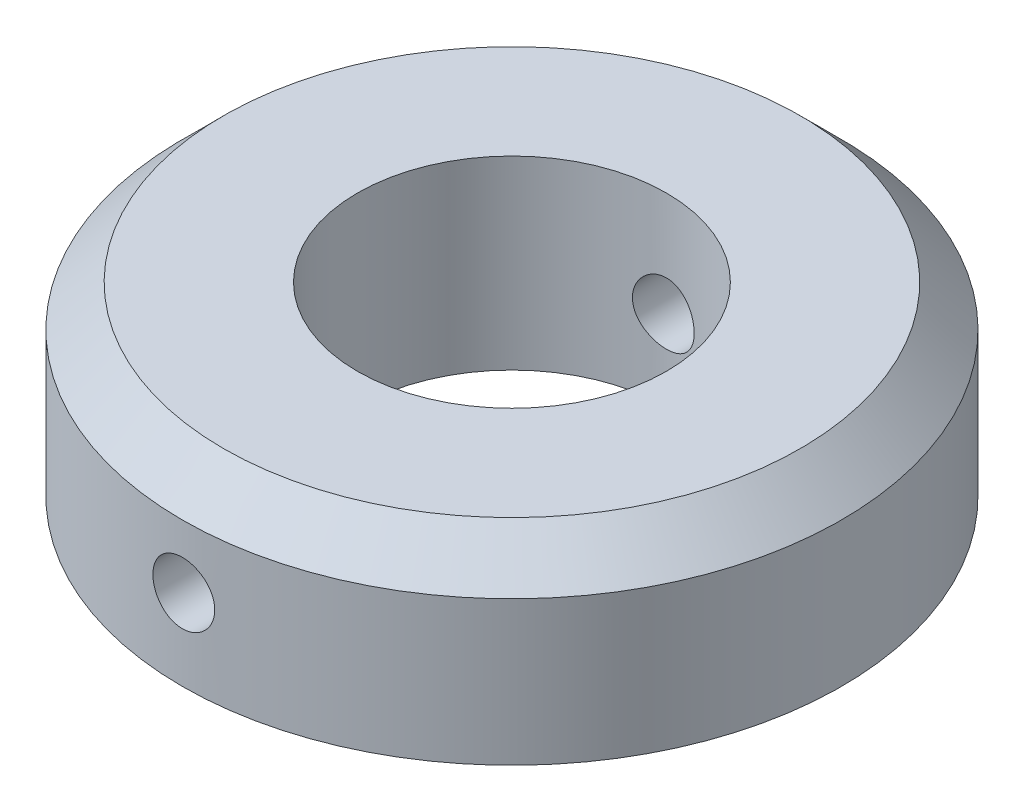
from build123d import *

# Parameters (mm, degrees)
COLLAR_RING_PROFILE_R   = 16
COLLAR_RING_PROFILE_R_2 = 7.5
COLLAR_BODY_DEPTH       = 9
EDGE_CHAMFER_2X45_SIZE  = 2
CROSS_HOLE_3_DEPTH      = 25.351591324
CROSS_HOLE_3_DEPTH_BACK = 25.351591324
CROSS_HOLE_PROFILE_R    = 1.5


with BuildPart() as part:
    # Collar Ring Profile → Collar Body (new body)
    with BuildSketch(Plane(origin=(0, 0, 0), x_dir=(1, 0, 0), z_dir=(0, 1, 0))):
        with Locations(Location((0, 0, 0), (0, 0, 270))):
            Circle(COLLAR_RING_PROFILE_R)
        with Locations(Location((0, 0, 0), (0, 0, 270))):
            Circle(COLLAR_RING_PROFILE_R_2, mode=Mode.SUBTRACT)
    extrude(amount=COLLAR_BODY_DEPTH)

    # Edge Chamfer 2x45
    edge_chamfer_2x45_edges = [part.edges().sort_by_distance(p)[0] for p in [
        (0, 9, -16),
    ]]
    chamfer(edge_chamfer_2x45_edges, length=EDGE_CHAMFER_2X45_SIZE)

    # Cross Hole Profile → Cross Hole Ø3 (cut, two sides: drawn at the far end of the back side and taken through both)
    with BuildSketch(Plane.XY.offset(-CROSS_HOLE_3_DEPTH_BACK)):
        with Locations((0, 3.930345363)):
            Circle(CROSS_HOLE_PROFILE_R)
    extrude(amount=CROSS_HOLE_3_DEPTH + CROSS_HOLE_3_DEPTH_BACK, mode=Mode.SUBTRACT)


solid = part.part
